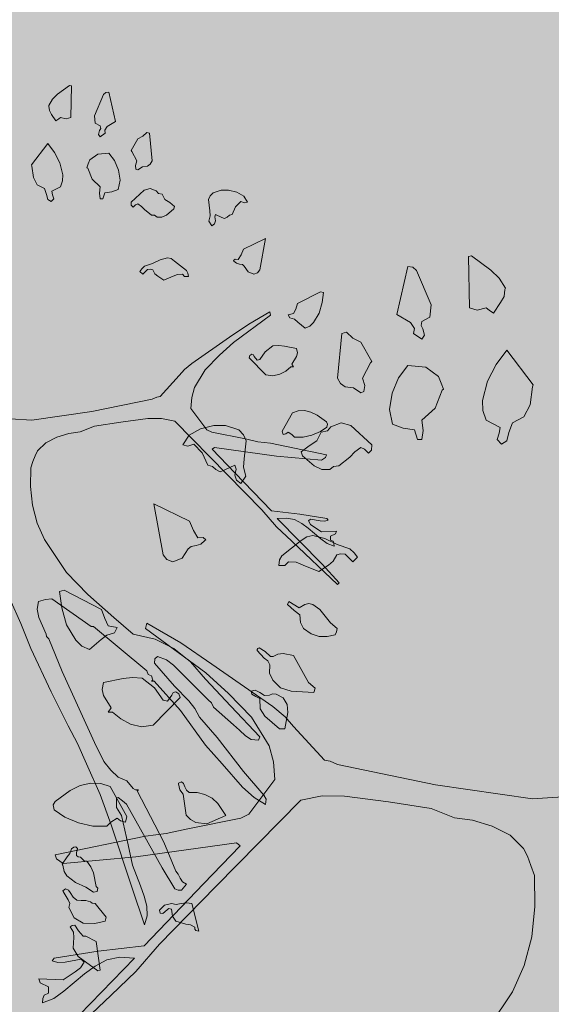
# Model space of a CAD drawing. Units: inches. Extents: x 84 to 1044, y -280 to 906.
# Tile 32 of 105: x 809 to 822, y -108 to -84. Entities that reach past the tile are written whole.
import ezdxf

# ---------------------------------------------------------------- set-up
doc = ezdxf.new("R2010")
doc.units = ezdxf.units.IN
doc.layers.add('L-PLNT', color=114, linetype='Continuous', lineweight=15)
doc.layers.add('L-PLNT-PATT', color=9, linetype='Continuous', lineweight=9, true_color=0xafd9aa)

# ---------------------------------------------------------------- blocks, each defined once
blk = doc.blocks.new('A$C37E508DF')
for p, q in [((0.96862, 1.43345), (0.98749, 1.44759)), ((0.98749, 1.44759), (0.99049, 1.44674)), ((0.99049, 1.44674), (0.98963, 1.39658)), ((0.96047, 1.42572), (0.96862, 1.43345)), ((1.02694, 1.39956), (1.04109, 1.43301)), ((1.04109, 1.43301), (1.04495, 1.43645)), ((1.04495, 1.43645), (1.04966, 1.43687)), ((1.04966, 1.43687), (1.06039, 1.39013)), ((0.95447, 1.41586), (0.96047, 1.42572)), ((0.95491, 1.41458), (0.95447, 1.41586)), ((0.95577, 1.40771), (0.95491, 1.41458)), ((0.95919, 1.40171), (0.95577, 1.40771)), ((0.96604, 1.39143), (0.95919, 1.40171)), ((0.97033, 1.39442), (0.96604, 1.39143)), ((0.97333, 1.39658), (0.97033, 1.39442)), ((0.98192, 1.39442), (0.97333, 1.39658)), ((0.98963, 1.39658), (0.98192, 1.39442)), ((1.02823, 1.38756), (1.02694, 1.39956)), ((1.03594, 1.38328), (1.02823, 1.38756)), ((1.06039, 1.39013), (1.04709, 1.38242)), ((1.03337, 1.36998), (1.03508, 1.37599)), ((1.03508, 1.37599), (1.0368, 1.37941)), ((1.0368, 1.37941), (1.03594, 1.38328)), ((1.04709, 1.38242), (1.04323, 1.37641)), ((1.04323, 1.37641), (1.04409, 1.3717)), ((1.03594, 1.36612), (1.03337, 1.36998)), ((1.04409, 1.3717), (1.03594, 1.36612)), ((1.09554, 1.36313), (1.10327, 1.36698)), ((1.10327, 1.36698), (1.1097, 1.37298)), ((1.1097, 1.37298), (1.11399, 1.3717)), ((1.11399, 1.3717), (1.11827, 1.32796)), ((1.08483, 1.34426), (1.09554, 1.36313)), ((0.92745, 1.32153), (0.95318, 1.3554)), ((0.95318, 1.3554), (0.96348, 1.34126)), ((0.96348, 1.34126), (0.97205, 1.32496)), ((1.01965, 1.32968), (1.03209, 1.33868)), ((1.03209, 1.33868), (1.04966, 1.3404)), ((1.04966, 1.3404), (1.05867, 1.32838)), ((1.08611, 1.34296), (1.08483, 1.34426)), ((1.09384, 1.32796), (1.08611, 1.34296)), ((1.01707, 1.32324), (1.01965, 1.32968)), ((1.05867, 1.32838), (1.0651, 1.31338)), ((1.09169, 1.32067), (1.09384, 1.32796)), ((1.11827, 1.32796), (1.11527, 1.32281)), ((0.92789, 1.31939), (0.92745, 1.32153)), ((0.93045, 1.30181), (0.92789, 1.31939)), ((0.97205, 1.32496), (0.97678, 1.30609)), ((1.01493, 1.31725), (1.01707, 1.32324)), ((1.09254, 1.3151), (1.09169, 1.32067)), ((1.10283, 1.31853), (1.09554, 1.3138)), ((1.11098, 1.31939), (1.10283, 1.31853)), ((1.11527, 1.32281), (1.11098, 1.31939)), ((1.01621, 1.31639), (1.01493, 1.31725)), ((1.02308, 1.2988), (1.01621, 1.31639)), ((1.0651, 1.31338), (1.06768, 1.29752)), ((1.09554, 1.3138), (1.09254, 1.3151)), ((0.93646, 1.29023), (0.93045, 1.30181)), ((0.97678, 1.30609), (0.97634, 1.29624)), ((1.03594, 1.2868), (1.02308, 1.2988)), ((0.94762, 1.28422), (0.93646, 1.29023)), ((0.97634, 1.29624), (0.97333, 1.2868)), ((1.06768, 1.29752), (1.06468, 1.28294)), ((0.95104, 1.27479), (0.94762, 1.28422)), ((0.97333, 1.2868), (0.95961, 1.27994)), ((0.95961, 1.27994), (0.96047, 1.27437)), ((1.03466, 1.27693), (1.03594, 1.2868)), ((1.05438, 1.27907), (1.04323, 1.27737)), ((1.06468, 1.28294), (1.05438, 1.27907)), ((1.08483, 1.26279), (1.10541, 1.28166)), ((1.10541, 1.28166), (1.11485, 1.28422)), ((1.11485, 1.28422), (1.1247, 1.28036)), ((1.1247, 1.28036), (1.12813, 1.27651)), ((1.21475, 1.27737), (1.22761, 1.28166)), ((1.22761, 1.28166), (1.2392, 1.28166)), ((1.2392, 1.28166), (1.25206, 1.27865)), ((0.95318, 1.26664), (0.95104, 1.27479)), ((0.96047, 1.27437), (0.96262, 1.26794)), ((1.03594, 1.26794), (1.03466, 1.27693)), ((1.04323, 1.27737), (1.04023, 1.26794)), ((1.12813, 1.27651), (1.13413, 1.27523)), ((1.13413, 1.27523), (1.13842, 1.26664)), ((1.20746, 1.26664), (1.21004, 1.27265)), ((1.21004, 1.27265), (1.21475, 1.27737)), ((1.25206, 1.27865), (1.26321, 1.27222)), ((1.26321, 1.27222), (1.2692, 1.26279)), ((0.95833, 1.26363), (0.95318, 1.26664)), ((0.96262, 1.26794), (0.95833, 1.26363)), ((1.04023, 1.26794), (1.03594, 1.26794)), ((1.08525, 1.25764), (1.08483, 1.26279)), ((1.09554, 1.26021), (1.09212, 1.2585)), ((1.10155, 1.25592), (1.09554, 1.26021)), ((1.13842, 1.26664), (1.14615, 1.26193)), ((1.14615, 1.26193), (1.15386, 1.25592)), ((1.2096, 1.24907), (1.20746, 1.26664)), ((1.25849, 1.26363), (1.25034, 1.25506)), ((1.26449, 1.26149), (1.25849, 1.26363)), ((1.2692, 1.26279), (1.26449, 1.26149)), ((1.08825, 1.25464), (1.08525, 1.25764)), ((1.09212, 1.2585), (1.08825, 1.25464)), ((1.10626, 1.25078), (1.10155, 1.25592)), ((1.11699, 1.2422), (1.10626, 1.25078)), ((1.15258, 1.25206), (1.141, 1.2422)), ((1.15386, 1.25592), (1.15258, 1.25206)), ((1.25034, 1.25506), (1.24477, 1.24306)), ((1.12214, 1.24178), (1.11699, 1.2422)), ((1.12598, 1.23878), (1.12214, 1.24178)), ((1.141, 1.2422), (1.13371, 1.23878)), ((1.2079, 1.23235), (1.21004, 1.24092)), ((1.21004, 1.24092), (1.2096, 1.24907)), ((1.21861, 1.24306), (1.21733, 1.2392)), ((1.22847, 1.23834), (1.21861, 1.24306)), ((1.24048, 1.24178), (1.23706, 1.23878)), ((1.24477, 1.24306), (1.24048, 1.24178)), ((1.13371, 1.23878), (1.12598, 1.23878)), ((1.2126, 1.22506), (1.2079, 1.23235)), ((1.21861, 1.23319), (1.21689, 1.22848)), ((1.21733, 1.2392), (1.21861, 1.23319)), ((1.23275, 1.23663), (1.22847, 1.23834)), ((1.23706, 1.23878), (1.23275, 1.23663)), ((1.21689, 1.22848), (1.2126, 1.22506)), ((1.26277, 1.18817), (1.2975, 1.20533)), ((1.2975, 1.20533), (1.28851, 1.15558)), ((1.25891, 1.17917), (1.26277, 1.18817)), ((1.13071, 1.17145), (1.14229, 1.17445)), ((1.14229, 1.17445), (1.14829, 1.17317)), ((1.14829, 1.17317), (1.15386, 1.1693)), ((1.25462, 1.17188), (1.25891, 1.17917)), ((1.10626, 1.16115), (1.11869, 1.16546)), ((1.11869, 1.16546), (1.13071, 1.17145)), ((1.15386, 1.1693), (1.17273, 1.1543)), ((1.24691, 1.17016), (1.24948, 1.17231)), ((1.24777, 1.1693), (1.24691, 1.17016)), ((1.25162, 1.16588), (1.24777, 1.1693)), ((1.24948, 1.17231), (1.25462, 1.17188)), ((1.25634, 1.16459), (1.25162, 1.16588)), ((1.26105, 1.16373), (1.25634, 1.16459)), ((1.26406, 1.16115), (1.26105, 1.16373)), ((1.09897, 1.15302), (1.10197, 1.1573)), ((1.10197, 1.1573), (1.10626, 1.16115)), ((1.11098, 1.15602), (1.10327, 1.14873)), ((1.11527, 1.15644), (1.11098, 1.15602)), ((1.11913, 1.15558), (1.11527, 1.15644)), ((1.12256, 1.14915), (1.11913, 1.15558)), ((1.17273, 1.1543), (1.17487, 1.15044)), ((1.27006, 1.15216), (1.26406, 1.16115)), ((1.28851, 1.15558), (1.28506, 1.15088)), ((1.10327, 1.14873), (1.09897, 1.15302)), ((1.12728, 1.14529), (1.12256, 1.14915)), ((1.13672, 1.1393), (1.12728, 1.14529)), ((1.15172, 1.14529), (1.13672, 1.1393)), ((1.15857, 1.14829), (1.15172, 1.14529)), ((1.1663, 1.14873), (1.15857, 1.14829)), ((1.16972, 1.14487), (1.1663, 1.14873)), ((1.17573, 1.14487), (1.16972, 1.14487)), ((1.17487, 1.15044), (1.17573, 1.14487)), ((1.27907, 1.14873), (1.27006, 1.15216)), ((1.28506, 1.15088), (1.27907, 1.14873)), ((1.34853, 1.10199), (1.38498, 1.12085)), ((1.38498, 1.12085), (1.38969, 1.11957)), ((1.38969, 1.11957), (1.38755, 1.10371)), ((1.34553, 1.09342), (1.34853, 1.10199)), ((1.38755, 1.10371), (1.38284, 1.08699)), ((1.27135, 1.0694), (1.30437, 1.08869)), ((1.30437, 1.08869), (1.30565, 1.08354)), ((1.3421, 1.08613), (1.34553, 1.09342)), ((1.38284, 1.08699), (1.37383, 1.07197)), ((1.30565, 1.08354), (1.24691, 1.04024)), ((1.33353, 1.0844), (1.3421, 1.08613)), ((1.33609, 1.07926), (1.33353, 1.0844)), ((1.34338, 1.07711), (1.33609, 1.07926)), ((1.34897, 1.07283), (1.34338, 1.07711)), ((1.2409, 1.04882), (1.27135, 1.0694)), ((1.36055, 1.06297), (1.34897, 1.07283)), ((1.37383, 1.07197), (1.36784, 1.0664)), ((1.36784, 1.0664), (1.36055, 1.06297)), ((1.1813, 1.00722), (1.2409, 1.04882)), ((1.24691, 1.04024), (1.22462, 1.02009)), ((1.29708, 1.02566), (1.30908, 1.0351)), ((1.30908, 1.0351), (1.31851, 1.03552)), ((1.31851, 1.03552), (1.32752, 1.03467)), ((1.32752, 1.03467), (1.34681, 1.03081)), ((1.34681, 1.03081), (1.34811, 1.02394)), ((1.22462, 1.02009), (1.20231, 0.99692)), ((1.27178, 1.01623), (1.27307, 1.01966)), ((1.27307, 1.01966), (1.27607, 1.0218)), ((1.27607, 1.0218), (1.27864, 1.02094)), ((1.27864, 1.02094), (1.27993, 1.01837)), ((1.28851, 1.01365), (1.29708, 1.02566)), ((1.34811, 1.02394), (1.34681, 1.01795)), ((1.29836, 0.98921), (1.27178, 1.01623)), ((1.27993, 1.01837), (1.28422, 1.01237)), ((1.28422, 1.01237), (1.28851, 1.01365)), ((1.34681, 1.01795), (1.3391, 1.00594)), ((1.1693, 0.99736), (1.1813, 1.00722)), ((1.33782, 1.00165), (1.32967, 0.99522)), ((1.3421, 1.00165), (1.33782, 1.00165)), ((1.3391, 1.00594), (1.3421, 1.00165)), ((1.16115, 0.98793), (1.1693, 0.99736)), ((1.20231, 0.99692), (1.18516, 0.96906)), ((1.32967, 0.99522), (1.32023, 0.99007)), ((1.13113, 0.95491), (1.16115, 0.98793)), ((1.30952, 0.98749), (1.29836, 0.98921)), ((1.32023, 0.99007), (1.30952, 0.98749)), ((1.18516, 0.96906), (1.18088, 0.9532)), ((1.11827, 0.95062), (1.12556, 0.95405)), ((1.12556, 0.95405), (1.13113, 0.95491)), ((1.18088, 0.9532), (1.1796, 0.93604)), ((1.02266, 0.93089), (1.11827, 0.95062)), ((1.1796, 0.93604), (1.20489, 0.90217)), ((0.92789, 0.91717), (1.02266, 0.93089)), ((1.3241, 0.90003), (1.34038, 0.92919)), ((1.34038, 0.92919), (1.34939, 0.93219)), ((1.34939, 0.93219), (1.35925, 0.93261)), ((1.35925, 0.93261), (1.36954, 0.93003)), ((1.36954, 0.93003), (1.37941, 0.92532)), ((1.37941, 0.92532), (1.39399, 0.91461)), ((0.89358, 0.91932), (0.92789, 0.91717)), ((1.06852, 0.91417), (1.02694, 0.90774)), ((1.1114, 0.91976), (1.06852, 0.91417)), ((1.13327, 0.92018), (1.1114, 0.91976)), ((1.15428, 0.91589), (1.13327, 0.92018)), ((1.23706, 0.83141), (1.15428, 0.91589)), ((1.39399, 0.91461), (1.3957, 0.91117)), ((1.02694, 0.90774), (1.00421, 0.89875)), ((1.39484, 0.90646), (1.38456, 0.89917)), ((1.3957, 0.91117), (1.39484, 0.90646)), ((0.98663, 0.89616), (0.96734, 0.8906)), ((1.00421, 0.89875), (0.98663, 0.89616)), ((1.20489, 0.90217), (1.2126, 0.89831)), ((1.2126, 0.89831), (1.2662, 0.88759)), ((1.32538, 0.89444), (1.3241, 0.90003)), ((1.33009, 0.89574), (1.32538, 0.89444)), ((1.33353, 0.89831), (1.33009, 0.89574)), ((1.33954, 0.89444), (1.33353, 0.89831)), ((1.34338, 0.8906), (1.33954, 0.89444)), ((1.38456, 0.89917), (1.37126, 0.8936)), ((0.96734, 0.8906), (0.94976, 0.88158)), ((1.2662, 0.88759), (1.2855, 0.88331)), ((1.3571, 0.8906), (1.34338, 0.8906)), ((1.37126, 0.8936), (1.3571, 0.8906)), ((0.94976, 0.88158), (0.9369, 0.86873)), ((1.2855, 0.88331), (1.30565, 0.88072)), ((1.30565, 0.88072), (1.39399, 0.8623)), ((0.9369, 0.86873), (0.93304, 0.861)), ((1.21689, 0.87429), (1.21346, 0.87129)), ((1.21346, 0.87129), (1.24905, 0.834)), ((1.31509, 0.86057), (1.21689, 0.87429)), ((0.93304, 0.861), (0.92961, 0.852)), ((1.38626, 0.85415), (1.31509, 0.86057)), ((1.39269, 0.85843), (1.38626, 0.85415)), ((1.39399, 0.8623), (1.39269, 0.85843)), ((0.92961, 0.852), (0.92617, 0.84213)), ((0.92617, 0.84213), (0.92575, 0.81213)), ((1.29193, 0.77524), (1.23706, 0.83141)), ((1.24905, 0.834), (1.30693, 0.77353)), ((0.92575, 0.81213), (0.92875, 0.78253)), ((0.92875, 0.78253), (0.93604, 0.75423)), ((1.31509, 0.74866), (1.29193, 0.77524)), ((1.30693, 0.77353), (1.35196, 0.76839)), ((1.33095, 0.76238), (1.31637, 0.76152)), ((1.31637, 0.76152), (1.38712, 0.68906)), ((1.34338, 0.75981), (1.33095, 0.76238)), ((1.35496, 0.75381), (1.34338, 0.75981)), ((1.35196, 0.76839), (1.39484, 0.76152)), ((1.36868, 0.76067), (1.36569, 0.75767)), ((1.38412, 0.75767), (1.36868, 0.76067)), ((1.39484, 0.76152), (1.39698, 0.75895)), ((0.93604, 0.75423), (0.94762, 0.72851)), ((1.36525, 0.74609), (1.35496, 0.75381)), ((1.36569, 0.75767), (1.36912, 0.75209)), ((1.36912, 0.75209), (1.37427, 0.74824)), ((1.39141, 0.75723), (1.38412, 0.75767)), ((1.39698, 0.75895), (1.39141, 0.75723)), ((1.3391, 0.72551), (1.31509, 0.74866)), ((1.3854, 0.72937), (1.36525, 0.74609)), ((1.37427, 0.74824), (1.38626, 0.74051)), ((1.38626, 0.74051), (1.40986, 0.74137)), ((1.40986, 0.74137), (1.40857, 0.73751)), ((1.40857, 0.73751), (1.40042, 0.73366)), ((1.40042, 0.73366), (1.40042, 0.72723)), ((0.94762, 0.72851), (0.98277, 0.6762)), ((1.41156, 0.65689), (1.3391, 0.72551)), ((1.39528, 0.72208), (1.3854, 0.72937)), ((1.40641, 0.7178), (1.39528, 0.72208)), ((1.40042, 0.72723), (1.40471, 0.72551)), ((1.40471, 0.72551), (1.40599, 0.72208)), ((1.40599, 0.72208), (1.40641, 0.7178)), ((1.38712, 0.68906), (1.41414, 0.6599)), ((0.98277, 0.6762), (1.01621, 0.64147)), ((1.41414, 0.6599), (1.41156, 0.65689)), ((1.01621, 0.64147), (1.05739, 0.60502)), ((0.9103, 0.59559), (0.89316, 0.63418)), ((0.93818, 0.63032), (0.93604, 0.61788)), ((0.94932, 0.63332), (0.93818, 0.63032)), ((0.95961, 0.63418), (0.94932, 0.63332)), ((1.0218, 0.59044), (0.95961, 0.63418)), ((1.33267, 0.62517), (1.33481, 0.63032)), ((1.34296, 0.61616), (1.33267, 0.62517)), ((1.33481, 0.63032), (1.35111, 0.62002)), ((1.35111, 0.62002), (1.36011, 0.62559)), ((1.36011, 0.62559), (1.36612, 0.62689)), ((1.36612, 0.62689), (1.37254, 0.62517)), ((1.37254, 0.62517), (1.3837, 0.61746)), ((0.93604, 0.61788), (0.93904, 0.60502)), ((1.35196, 0.60887), (1.34296, 0.61616)), ((1.3837, 0.61746), (1.39185, 0.60716)), ((1.35326, 0.59687), (1.35196, 0.60887)), ((1.39185, 0.60716), (1.40042, 0.59643)), ((0.93904, 0.60502), (0.95062, 0.57842)), ((1.05739, 0.60502), (1.08825, 0.57842)), ((1.35796, 0.58744), (1.35326, 0.59687)), ((1.40042, 0.59643), (1.41114, 0.58744)), ((0.92617, 0.55571), (0.9103, 0.59559)), ((1.02565, 0.59044), (1.0218, 0.59044)), ((1.1097, 0.52054), (1.02565, 0.59044)), ((1.36998, 0.57886), (1.35796, 0.58744)), ((1.41114, 0.58744), (1.41028, 0.58229)), ((0.95062, 0.57842), (0.95104, 0.57458)), ((1.08825, 0.57842), (1.12298, 0.57027)), ((1.38242, 0.575), (1.36998, 0.57886)), ((1.40771, 0.57714), (1.39528, 0.57458)), ((1.41028, 0.58229), (1.40771, 0.57714)), ((0.95104, 0.57458), (0.95447, 0.57113)), ((0.95447, 0.57113), (0.97591, 0.51926)), ((1.12298, 0.57027), (1.15258, 0.55571)), ((1.39528, 0.57458), (1.38242, 0.575)), ((0.95833, 0.4871), (0.92617, 0.55571)), ((1.15258, 0.55571), (1.17916, 0.53468)), ((1.28422, 0.55399), (1.2855, 0.55571)), ((1.28422, 0.55271), (1.28422, 0.55399)), ((1.2958, 0.54069), (1.28422, 0.55271)), ((1.2855, 0.55571), (1.28765, 0.55699)), ((1.28765, 0.55699), (1.29708, 0.55099)), ((1.29708, 0.55099), (1.30565, 0.54327)), ((1.12256, 0.53941), (1.12214, 0.53254)), ((1.12684, 0.54327), (1.12256, 0.53941)), ((1.141, 0.53769), (1.12684, 0.54327)), ((1.30137, 0.53598), (1.2958, 0.54069)), ((1.30565, 0.54327), (1.30994, 0.54327)), ((1.30994, 0.54327), (1.31723, 0.5467)), ((1.31723, 0.5467), (1.32538, 0.54798)), ((1.32538, 0.54798), (1.3421, 0.54456)), ((1.3421, 0.54456), (1.36569, 0.5021)), ((1.12214, 0.53254), (1.15386, 0.49611)), ((1.15214, 0.52955), (1.141, 0.53769)), ((1.17058, 0.51111), (1.15214, 0.52955)), ((1.17916, 0.53468), (1.20275, 0.50725)), ((1.30437, 0.52998), (1.30137, 0.53598)), ((1.30393, 0.51668), (1.30437, 0.52998)), ((0.97591, 0.51926), (1.02694, 0.40691)), ((1.11184, 0.51454), (1.1097, 0.52054)), ((1.11699, 0.51239), (1.11184, 0.51454)), ((1.11913, 0.50554), (1.11699, 0.51239)), ((1.19546, 0.48581), (1.17058, 0.51111)), ((1.30908, 0.50554), (1.30393, 0.51668)), ((1.11699, 0.50424), (1.11913, 0.50554)), ((1.1217, 0.50424), (1.11699, 0.50424)), ((1.16329, 0.45752), (1.1217, 0.50424)), ((1.20275, 0.50725), (1.24262, 0.46437)), ((1.32151, 0.49353), (1.30908, 0.50554)), ((1.36569, 0.5021), (1.37641, 0.49267)), ((1.15386, 0.49611), (1.17615, 0.47294)), ((1.33824, 0.48838), (1.32151, 0.49353)), ((1.37641, 0.49267), (1.37427, 0.48581)), ((0.98535, 0.4335), (0.95833, 0.4871)), ((1.20703, 0.47466), (1.19546, 0.48581)), ((1.27479, 0.48838), (1.28122, 0.48966)), ((1.27607, 0.48323), (1.27479, 0.48838)), ((1.2825, 0.47981), (1.27607, 0.48323)), ((1.28122, 0.48966), (1.28851, 0.48624)), ((1.28851, 0.48624), (1.29622, 0.48153)), ((1.29622, 0.48153), (1.30393, 0.48195)), ((1.30393, 0.48195), (1.30866, 0.48409)), ((1.30866, 0.48409), (1.31466, 0.48323)), ((1.31466, 0.48323), (1.3258, 0.47766)), ((1.37427, 0.48581), (1.33824, 0.48838)), ((1.17615, 0.47294), (1.18559, 0.46052)), ((1.21218, 0.46995), (1.20703, 0.47466)), ((1.28851, 0.47638), (1.2825, 0.47981)), ((1.28937, 0.46008), (1.28851, 0.47638)), ((1.3258, 0.47766), (1.33181, 0.46695)), ((1.21561, 0.46266), (1.21218, 0.46995)), ((1.24691, 0.43478), (1.21561, 0.46266)), ((1.24262, 0.46437), (1.28851, 0.41592)), ((1.33181, 0.46695), (1.33309, 0.45451)), ((1.20275, 0.40262), (1.16329, 0.45752)), ((1.18559, 0.46052), (1.19332, 0.44678)), ((1.29666, 0.4485), (1.28937, 0.46008)), ((1.33309, 0.45451), (1.32838, 0.42836)), ((1.19332, 0.44678), (1.22118, 0.41464)), ((1.30823, 0.43865), (1.29666, 0.4485)), ((1.00035, 0.4052), (0.98535, 0.4335)), ((1.25677, 0.42663), (1.24691, 0.43478)), ((1.31981, 0.42836), (1.30823, 0.43865)), ((1.26578, 0.41764), (1.25677, 0.42663)), ((1.32838, 0.42836), (1.31981, 0.42836)), ((1.22118, 0.41464), (1.26277, 0.36102)), ((1.27521, 0.41163), (1.26578, 0.41764)), ((1.28851, 0.41592), (1.28679, 0.41077)), ((1.01451, 0.37304), (1.00035, 0.4052)), ((1.02694, 0.40691), (1.04195, 0.3769)), ((1.28679, 0.41077), (1.27521, 0.41163)), ((1.2289, 0.37304), (1.20275, 0.40262)), ((1.04195, 0.3769), (1.05266, 0.36317)), ((1.03594, 0.32459), (1.01451, 0.37304)), ((1.26149, 0.33617), (1.2289, 0.37304)), ((1.05266, 0.36317), (1.06468, 0.35203)), ((1.26277, 0.36102), (1.29494, 0.32329)), ((1.06468, 0.35203), (1.07796, 0.34602)), ((1.07796, 0.34602), (1.08825, 0.33402)), ((1.15987, 0.3426), (1.16458, 0.34474)), ((1.15987, 0.34131), (1.15987, 0.3426)), ((1.16201, 0.33188), (1.15987, 0.34131)), ((1.16458, 0.34474), (1.16802, 0.34174)), ((1.16802, 0.34174), (1.17016, 0.33659)), ((1.17016, 0.33659), (1.17273, 0.33144)), ((1.08825, 0.33402), (1.09212, 0.33188)), ((1.09212, 0.33188), (1.09682, 0.33188)), ((1.09682, 0.33188), (1.09468, 0.33058)), ((1.09468, 0.33058), (1.13672, 0.24911)), ((1.16758, 0.32501), (1.16201, 0.33188)), ((1.17273, 0.33144), (1.17701, 0.32758)), ((1.17701, 0.32758), (1.18945, 0.32758)), ((1.18945, 0.32758), (1.20189, 0.32459)), ((1.2795, 0.31987), (1.26149, 0.33617)), ((1.05352, 0.27656), (1.03594, 0.32459)), ((1.06468, 0.31987), (1.06167, 0.31944)), ((1.06167, 0.31944), (1.06167, 0.304)), ((1.07111, 0.31472), (1.06468, 0.31987)), ((1.17187, 0.29199), (1.16758, 0.32501)), ((1.20189, 0.32459), (1.21346, 0.31858)), ((1.21346, 0.31858), (1.22248, 0.31043)), ((1.2975, 0.30871), (1.2795, 0.31987)), ((1.29494, 0.32329), (1.2988, 0.3173)), ((1.07754, 0.30915), (1.07111, 0.31472)), ((1.13413, 0.20837), (1.07754, 0.30915)), ((1.22248, 0.31043), (1.2349, 0.29114)), ((1.2988, 0.3173), (1.2975, 0.30871)), ((1.06167, 0.304), (1.06982, 0.29114)), ((1.06982, 0.29114), (1.08054, 0.24482)), ((1.17916, 0.2847), (1.17187, 0.29199)), ((1.2349, 0.29114), (1.20489, 0.27827)), ((1.18731, 0.27999), (1.17916, 0.2847)), ((1.20489, 0.27827), (1.18731, 0.27999)), ((1.08611, 0.17751), (1.05352, 0.27656)), ((0.99049, 0.23839), (0.99434, 0.24098)), ((0.99434, 0.24098), (0.99735, 0.2414)), ((0.99735, 0.2414), (1.00035, 0.23925)), ((1.08054, 0.24482), (1.08697, 0.21268)), ((1.13672, 0.24911), (1.15558, 0.20324)), ((0.98363, 0.22596), (0.98791, 0.2311)), ((0.98791, 0.2311), (0.99049, 0.23839)), ((1.00035, 0.23925), (0.99865, 0.23196)), ((0.99865, 0.23196), (0.99865, 0.2281)), ((0.97591, 0.21396), (0.98363, 0.22596)), ((0.99865, 0.2281), (1.00121, 0.22553)), ((1.00121, 0.22553), (1.00507, 0.2251)), ((1.00507, 0.2251), (1.00764, 0.22253)), ((1.00764, 0.22253), (1.01064, 0.21953)), ((0.97678, 0.21268), (0.97591, 0.21396)), ((0.97892, 0.2028), (0.97678, 0.21268)), ((1.01064, 0.21953), (1.01493, 0.21911)), ((1.01493, 0.21911), (1.02136, 0.21009)), ((1.08697, 0.21268), (1.09983, 0.17965)), ((0.9832, 0.19551), (0.97892, 0.2028)), ((1.02136, 0.21009), (1.02522, 0.20024)), ((1.15428, 0.17493), (1.13413, 0.20837)), ((1.15558, 0.20324), (1.15943, 0.19852)), ((0.99692, 0.18522), (0.9832, 0.19551)), ((1.02522, 0.20024), (1.02951, 0.17879)), ((1.15943, 0.19852), (1.16243, 0.19209)), ((1.01321, 0.17793), (0.99692, 0.18522)), ((1.16243, 0.19209), (1.1663, 0.18608)), ((1.1663, 0.18608), (1.17273, 0.18266)), ((0.97678, 0.17194), (0.98106, 0.17493)), ((0.98106, 0.17493), (0.98577, 0.17278)), ((1.02565, 0.1698), (1.01321, 0.17793)), ((1.02951, 0.17879), (1.03251, 0.17623)), ((1.03251, 0.17623), (1.03123, 0.17108)), ((1.10626, 0.11833), (1.08611, 0.17751)), ((1.09983, 0.17965), (1.10584, 0.16335)), ((1.15943, 0.17278), (1.15428, 0.17493)), ((1.16458, 0.17322), (1.15943, 0.17278)), ((1.17273, 0.18266), (1.16458, 0.17322)), ((0.97762, 0.17108), (0.97678, 0.17194)), ((0.98535, 0.15778), (0.97762, 0.17108)), ((0.98577, 0.17278), (0.98835, 0.16936)), ((0.98835, 0.16936), (0.99306, 0.16165)), ((1.03123, 0.17108), (1.02565, 0.1698)), ((0.98791, 0.15177), (0.98535, 0.15778)), ((0.99306, 0.16165), (0.99907, 0.15736)), ((0.99907, 0.15736), (1.00594, 0.1565)), ((1.00594, 0.1565), (1.01321, 0.1565)), ((1.01321, 0.1565), (1.0205, 0.15478)), ((1.0205, 0.15478), (1.0235, 0.15221)), ((1.10584, 0.16335), (1.1097, 0.14749)), ((0.98663, 0.14534), (0.98791, 0.15177)), ((0.99478, 0.12906), (0.98663, 0.14534)), ((1.0235, 0.15221), (1.02823, 0.15177)), ((1.02823, 0.15177), (1.04537, 0.13034)), ((1.1097, 0.14749), (1.11012, 0.13249)), ((1.12985, 0.14106), (1.13756, 0.14921)), ((1.13756, 0.14921), (1.14914, 0.15177)), ((1.14914, 0.15177), (1.15643, 0.15049)), ((1.15643, 0.15049), (1.16416, 0.15177)), ((1.16416, 0.15177), (1.17273, 0.15307)), ((1.17273, 0.15307), (1.1813, 0.15177)), ((1.1813, 0.15177), (1.19202, 0.10803)), ((1.13113, 0.13635), (1.12985, 0.14106)), ((1.13542, 0.13591), (1.13113, 0.13635)), ((1.13842, 0.13892), (1.13542, 0.13591)), ((1.14229, 0.14234), (1.13842, 0.13892)), ((1.14485, 0.14406), (1.14229, 0.14234)), ((1.14914, 0.14278), (1.14485, 0.14406)), ((1.15044, 0.13205), (1.14914, 0.14278)), ((1.00892, 0.12047), (0.99478, 0.12906)), ((1.04537, 0.13034), (1.04409, 0.12391)), ((1.11012, 0.13249), (1.10626, 0.11833)), ((1.15558, 0.12391), (1.15044, 0.13205)), ((0.98835, 0.1149), (0.99178, 0.11705)), ((0.99178, 0.11705), (0.99606, 0.11748)), ((0.99606, 0.11748), (1.00163, 0.10847)), ((1.02737, 0.12005), (1.00892, 0.12047)), ((1.04409, 0.12391), (1.02737, 0.12005)), ((1.17145, 0.11919), (1.15558, 0.12391)), ((1.17916, 0.11791), (1.17145, 0.11919)), ((1.18603, 0.11448), (1.17916, 0.11791)), ((0.9935, 0.10633), (0.98835, 0.1149)), ((0.99434, 0.09818), (0.9935, 0.10633)), ((1.00163, 0.10847), (1.00892, 0.0999)), ((1.18559, 0.11104), (1.18603, 0.11448)), ((1.18731, 0.10933), (1.18559, 0.11104)), ((1.19202, 0.10803), (1.18731, 0.10933)), ((0.99306, 0.08103), (0.99434, 0.09818)), ((1.00892, 0.0999), (1.01321, 0.0999)), ((1.01321, 0.0999), (1.02951, 0.09175)), ((1.02951, 0.09175), (1.03594, 0.04629)), ((1.00121, 0.06774), (0.99306, 0.08103)), ((1.03251, 0.04544), (1.00121, 0.06774)), ((1.03594, 0.04629), (1.03251, 0.04544))]:
    blk.add_line(p, q)

msp = doc.modelspace()

# ---------------------------------------------------------------- hatches: boundary and pattern name
at = {"layer": 'L-PLNT-PATT', "transparency": 33554597}
h = msp.add_hatch(color=256, dxfattribs=at)
h.dxf.hatch_style = 1
h.paths.add_polyline_path([(791.074, 31.12), (791.074, 91.12), (743.074, 91.12), (674.074, 91.12), (674.074, 31.12), (650.074, 31.12), (650.074, -112.88), (983.074, -112.88), (983.074, -64.88), (791.074, -64.88)])

# ---------------------------------------------------------------- block references
at = {"layer": 'L-PLNT'}
for p, xscale, yscale, zscale in [((795.564, -107.745), 15.19586232982809, 15.19586232982809, 15.19586232982809), ((844.575, -125.52), -24.64361536662419, 24.64361536662419, 24.64361536662419)]:
    msp.add_blockref('A$C37E508DF', p, dxfattribs=dict(at, xscale=xscale, yscale=yscale, zscale=zscale))

doc.saveas('drawing.dxf')
